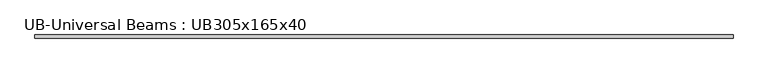
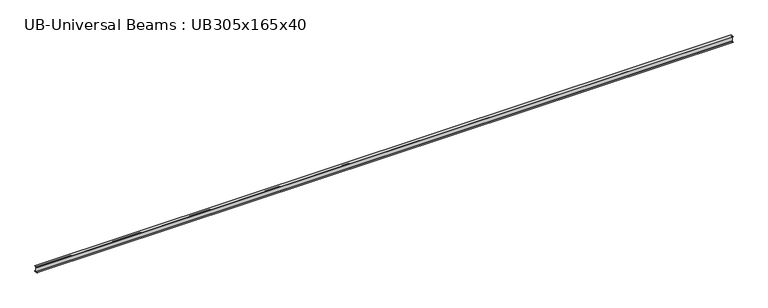
"""IFC4 building model written with IfcOpenShell, lengths in millimetres: beam geometry, UB-Universal Beams : UB305x165x40."""

from ifc_helpers import new_model, si_unit, point, frame, frame_2d, origin, place, context, project, spatial, polyline, circle_curve, trimmed, segment, composite_curve, outline, extrude, source, transform, mapped, element, save


def ub_universal_beams_ub305x165x40_a59d1a35(model_context):
    return source(origin(), model_context, "Body", "SweptSolid", [
        extrude(outline(composite_curve([segment(polyline([(82.5, -141.5), (82.5, -151.7), (-82.5, -151.7), (-82.5, -141.5), (-11.9, -141.5)]), True, "CONTINUOUS"), segment(trimmed(circle_curve(frame_2d((-11.9, -132.6)), 8.9), [point((-11.9, -141.5))], [point((-3.0, -132.6))], True, "CARTESIAN"), True, "CONTINUOUS"), segment(polyline([(-3.0, -132.6), (-3.0, 132.6)]), True, "CONTINUOUS"), segment(trimmed(circle_curve(frame_2d((-11.9, 132.6)), 8.9), [point((-3.0, 132.6))], [point((-11.9, 141.5))], True, "CARTESIAN"), True, "CONTINUOUS"), segment(polyline([(-11.9, 141.5), (-82.5, 141.5), (-82.5, 151.7), (82.5, 151.7), (82.5, 141.5), (11.9, 141.5)]), True, "CONTINUOUS"), segment(trimmed(circle_curve(frame_2d((11.9, 132.6)), 8.9), [point((11.9, 141.5))], [point((3.0, 132.6))], True, "CARTESIAN"), True, "CONTINUOUS"), segment(polyline([(3.0, 132.6), (3.0, -132.6)]), True, "CONTINUOUS"), segment(trimmed(circle_curve(frame_2d((11.9, -132.6)), 8.9), [point((3.0, -132.6))], [point((11.9, -141.5))], True, "CARTESIAN"), True, "CONTINUOUS"), segment(polyline([(11.9, -141.5), (82.5, -141.5)]), True, "CONTINUOUS")], self_intersect=False)), frame((-18192.8, 0.0, 0.0), z_axis=(1.0, 0.0, 0.0), x_axis=(0.0, 1.0, 0.0)), (0.0, 0.0, 1.0), 36385.6),
    ])


if __name__ == "__main__":
    model = new_model("IFC4")
    model_context = context("Model", 3, world=origin())
    ifc_project = project(units=[si_unit("LENGTHUNIT", "METRE", prefix="MILLI")], contexts=[model_context])
    site = spatial("IfcSite", under=ifc_project)
    building = spatial("IfcBuilding", under=site)
    placement = place(None, origin())
    ub_universal_beams_ub305x165x40_shape = ub_universal_beams_ub305x165x40_a59d1a35(model_context)
    element("IfcBeam", 1, ObjectType="UB-Universal Beams : UB305x165x40", at=placement, inside=building, context=model_context, shape_type="MappedRepresentation", body=[
        mapped(ub_universal_beams_ub305x165x40_shape, transform((0.0, 0.0, 0.0), x_axis=(1.0, 0.0, 0.0), y_axis=(0.0, 1.0, 0.0), z_axis=(0.0, 0.0, 1.0))),
    ])
    save(model, "model.ifc")

# Revit data of these elements
# Type "UB-Universal Beams : UB305x165x40"
#   Section Name Key = "UB305X165X40"
#   Width = 16.5 cm
#   Web Thickness = 0.6 cm
#   Web Fillet = 0.89 cm
#   Warping Constant = 164000.0 cm⁶
#   Torsional Moment of Inertia = 14.70 cm⁴
#   Section Area = 51.3 cm²
#   Plastic Modulus weak axis = 142.0 cm³
#   Plastic Modulus strong axis = 623.0 cm³
#   Nominal Weight = 40.2999 kgf/m
#   Moment of Inertia weak axis = 764.00 cm⁴
#   Moment of Inertia strong axis = 8503.00 cm⁴
#   Height = 30.34 cm
#   Flange Thickness = 1.02 cm
#   Elastic Modulus weak axis = 92.6 cm³
#   Elastic Modulus strong axis = 560.0 cm³
#   Centroid Vertical = 15.17 cm
#   Centroid Horizontal = 8.25 cm
#   Bolt Spacing = 9.0 cm
#   Length [instance default] = 1500 mm
#   Structural Material [instance default] = Metal - Steel 43-275
#   Type Comments = ""
#   Assembly Code = ""
# Element 1 (IfcBeam, "UB-Universal Beams : UB305x165x40")
#   Materials on its faces: "Metal - Steel 43-275"
# Materials
#   "Metal - Steel 43-275": class "Metal", colour RGB 247 247 247, transparency 0, Cost = 0
